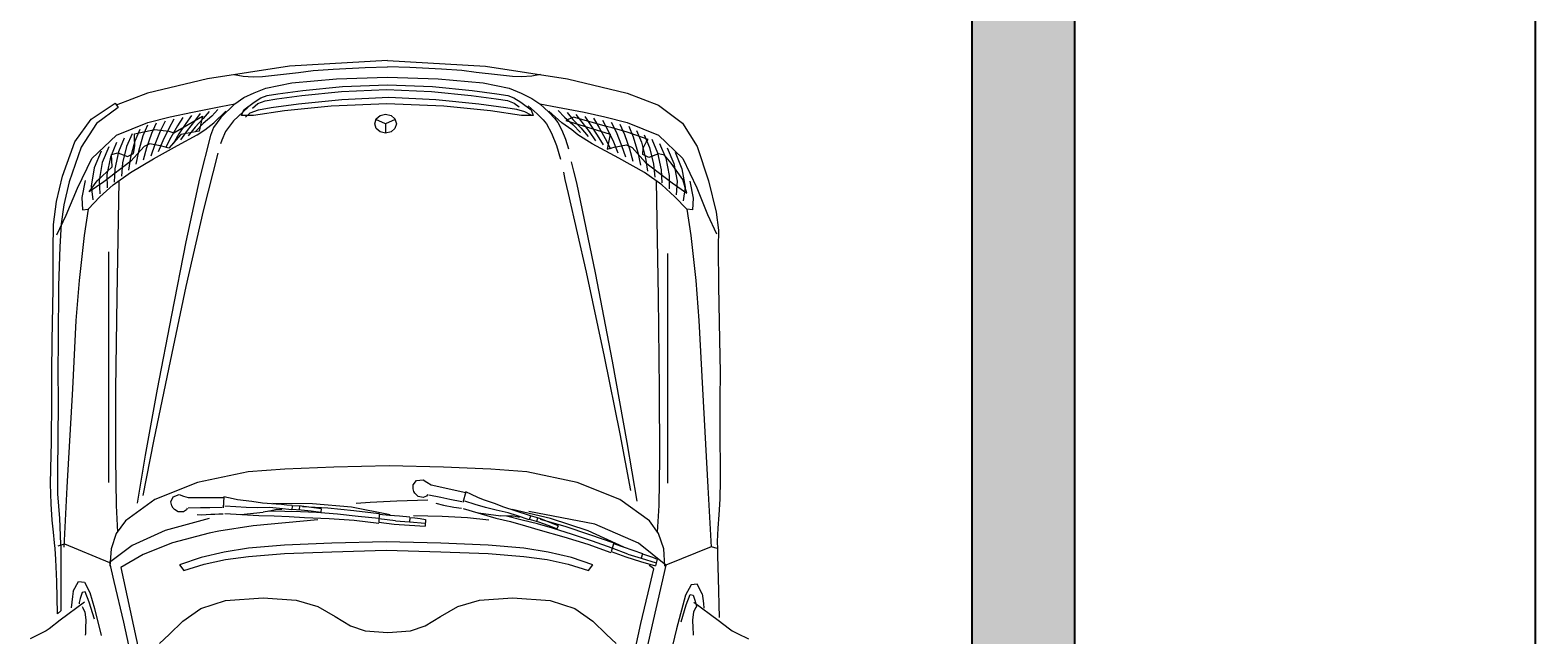
# Model space of a CAD drawing. Units: inches. Extents: x -9 to 646, y -802 to 47.
# Tile 12 of 17: x 517 to 646, y -576 to -524. Entities that reach past the tile are written whole.
import ezdxf

# ---------------------------------------------------------------- set-up
doc = ezdxf.new("R2010")
doc.units = ezdxf.units.IN
doc.header["$MEASUREMENT"] = 0
for name, color, linetype, lineweight in [('A-ANNO-DIMS', 2, 'Continuous', 18), ('A-SITE-VEHI', 8, 'Continuous', 9), ('A-WALL-PATT', 5, 'Continuous', 9), ('C-SITE', 7, 'Continuous', 25)]:
    doc.layers.add(name, color=color, linetype=linetype, lineweight=lineweight)
doc.styles.get("Standard").update_dxf_attribs({"font": 'arial.ttf'})
doc.dimstyles.get("Standard").update_dxf_attribs({"dimtxt": 0.18, "dimasz": 0.18, "dimexe": 0.18, "dimexo": 0.0625, "dimgap": 0.09, "dimtad": 0, "dimtih": 1, "dimtoh": 1, "dimdec": 0, "dimzin": 0, "dimdsep": 46, "dimlunit": 3, "dimtxsty": 'Standard', "dimcen": 0.09, "dimadec": 0, "dimazin": 0, "dimtfac": 1, "dimtdec": 0, "dimtofl": 0, "dimtmove": 0, "dimatfit": 3, "dimfxl": 1, "dimtolj": 1, "dimtzin": 0, "dimarcsym": 0})

# ---------------------------------------------------------------- blocks, each defined once
blk = doc.blocks.new('*D50')
at = {"layer": 'A-ANNO-DIMS', "color": 0, "lineweight": -2, "transparency": 16777216}
for p, q in [((606.44, 7.93), (645.8, 7.93)), ((645.62, 7.75), (645.62, -376.89)), ((645.62, -761.89), (645.62, -377.25)), ((606.44, -762.07), (645.8, -762.07))]:
    blk.add_line(p, q, dxfattribs=at)
at = {"layer": 'A-ANNO-DIMS', "color": 0, "transparency": 16777216}
for points in [[(645.59, 7.75), (645.65, 7.75), (645.62, 7.93)], [(645.59, -761.89), (645.65, -761.89), (645.62, -762.07)]]:
    blk.add_solid(points, dxfattribs=at)
at = {"layer": 'Defpoints', "color": 0, "transparency": 16777216}
for p in [(606.37, 7.93), (606.37, -762.07), (645.62, -762.07)]:
    blk.add_point(p, dxfattribs=at)
at = {"layer": 'A-ANNO-DIMS', "color": 0, "transparency": 16777216, "insert": (645.62, -377.07), "char_height": 0.18, "attachment_point": 5}
blk.add_mtext('\\A1;770', dxfattribs=at)

msp = doc.modelspace()

# ---------------------------------------------------------------- hatches: boundary and pattern name
at = {"layer": 'A-WALL-PATT'}
h = msp.add_hatch(color=256, dxfattribs=at)
h.dxf.hatch_style = 1
h.paths.add_polyline_path([(597.63, -101.57), (570.37, -101.57), (570.37, -496.07), (570.37, -511.17), (597.63, -511.17)], flags=0)
h.paths.add_polyline_path([(606.37, -101.57), (597.63, -101.57), (597.63, -511.17), (570.37, -511.17), (570.37, -513.2), (597.63, -513.2), (597.63, -712.07), (606.37, -712.07)])

# ---------------------------------------------------------------- linework, layer by layer
at = {"layer": 'A-SITE-VEHI'}
for p, q in [((539.54, -527.27), (532.56, -528.33)), ((547.88, -526.77), (539.54, -527.27)), ((541.55, -527.64), (543.27, -527.51)), ((543.27, -527.51), (545.99, -527.38)), ((545.99, -527.38), (547.88, -527.32)), ((547.88, -526.77), (556.22, -527.27)), ((549.78, -527.38), (547.88, -527.32)), ((552.5, -527.51), (549.78, -527.38)), ((554.21, -527.64), (552.5, -527.51)), ((556.22, -527.27), (563.21, -528.33)), ((532.56, -528.33), (527.46, -529.57)), ((534.84, -527.97), (535.59, -528.12)), ((535.59, -528.12), (536.46, -528.16)), ((536.46, -528.16), (537.24, -528.13)), ((537.24, -528.13), (538.52, -528.01)), ((537.52, -529.12), (539.73, -528.68)), ((538.52, -528.01), (540.31, -527.81)), ((539.73, -528.68), (543.56, -528.33)), ((540.31, -527.81), (541.55, -527.64)), ((543.56, -528.33), (547.88, -528.19)), ((544.05, -529), (547.88, -528.84)), ((547.88, -528.19), (552.21, -528.33)), ((547.88, -528.84), (551.72, -529)), ((552.21, -528.33), (556.04, -528.68)), ((555.45, -527.81), (554.21, -527.64)), ((557.25, -528.01), (555.45, -527.81)), ((556.04, -528.68), (558.25, -529.12)), ((558.52, -528.13), (557.25, -528.01)), ((559.3, -528.16), (558.52, -528.13)), ((560.18, -528.12), (559.3, -528.16)), ((560.92, -527.97), (560.18, -528.12)), ((563.21, -528.33), (568.3, -529.57)), ((527.46, -529.57), (524.8, -530.59)), ((534.9, -530.48), (535.65, -529.93)), ((535.65, -529.93), (536.53, -529.52)), ((536.53, -529.52), (537.52, -529.12)), ((536.53, -530.32), (537.11, -529.96)), ((537.11, -529.96), (537.64, -529.76)), ((537.47, -530.2), (538.47, -530.03)), ((537.64, -529.76), (538.55, -529.61)), ((538.47, -530.03), (540.6, -529.76)), ((538.55, -529.61), (540.68, -529.34)), ((540.3, -530.47), (543.99, -530.09)), ((540.6, -529.76), (543.96, -529.42)), ((540.68, -529.34), (544.05, -529)), ((543.96, -529.42), (547.8, -529.26)), ((543.99, -530.09), (548.01, -529.89)), ((547.8, -529.26), (551.64, -529.42)), ((548.01, -529.89), (552.01, -530.09)), ((551.64, -529.42), (555, -529.76)), ((551.72, -529), (555.09, -529.34)), ((552.01, -530.09), (555.66, -530.47)), ((555, -529.76), (557.13, -530.03)), ((555.09, -529.34), (557.21, -529.61)), ((557.13, -530.03), (558.1, -530.19)), ((557.21, -529.61), (558.13, -529.76)), ((558.13, -529.76), (558.65, -529.96)), ((558.25, -529.12), (559.27, -529.56)), ((558.65, -529.96), (559.23, -530.32)), ((559.27, -529.56), (560.17, -530.01)), ((560.17, -530.01), (560.87, -530.48)), ((568.3, -529.57), (570.96, -530.59)), ((522.67, -531.77), (524.69, -530.4)), ((524.95, -530.78), (523.1, -532.15)), ((524.69, -530.4), (524.95, -530.78)), ((529.39, -531.57), (531.3, -531.17)), ((531.3, -531.17), (533.71, -530.7)), ((531.95, -531.29), (531.46, -531.93)), ((532.7, -531.12), (532.19, -531.72)), ((533.45, -530.96), (532.92, -531.51)), ((533.11, -532.08), (534.13, -531.08)), ((534.9, -530.48), (533.69, -531.64)), ((533.71, -530.7), (534.9, -530.48)), ((536.04, -530.76), (534.77, -531.92)), ((535.46, -531.46), (535.66, -530.98)), ((535.66, -530.98), (536.53, -530.32)), ((535.81, -531.59), (536.19, -531.24)), ((536.19, -531.24), (536.91, -530.97)), ((536.39, -530.84), (536.85, -530.44)), ((539.12, -531.06), (536.48, -531.46)), ((536.85, -530.44), (537.47, -530.2)), ((536.91, -530.97), (537.99, -530.77)), ((537.99, -530.77), (540.3, -530.47)), ((543.09, -530.66), (539.12, -531.06)), ((547.83, -530.48), (543.09, -530.66)), ((547.26, -531.45), (547.72, -531.34)), ((547.72, -531.34), (548.19, -531.45)), ((552.69, -530.66), (547.83, -530.48)), ((556.66, -531.06), (552.69, -530.66)), ((555.66, -530.47), (557.95, -530.77)), ((559.29, -531.46), (556.66, -531.06)), ((557.95, -530.77), (558.88, -530.92)), ((558.1, -530.19), (558.68, -530.4)), ((558.68, -530.4), (559.11, -530.71)), ((558.88, -530.92), (559.54, -531.11)), ((559.23, -530.32), (560.11, -530.98)), ((559.54, -531.11), (560.09, -531.4)), ((559.86, -530.63), (560.62, -531.32)), ((560.11, -530.98), (560.3, -531.46)), ((560.62, -531.32), (561.13, -531.82)), ((560.87, -530.48), (561.62, -531.18)), ((560.87, -530.48), (562.36, -530.74)), ((561.62, -531.18), (562.12, -531.69)), ((562.73, -532.08), (561.63, -531.08)), ((562.36, -530.74), (564.62, -531.19)), ((562.43, -531.04), (562.95, -531.59)), ((563.18, -531.21), (563.68, -531.81)), ((563.93, -531.37), (564.42, -532.02)), ((564.62, -531.19), (566.38, -531.57)), ((570.96, -530.59), (573, -532.11)), ((521.28, -533.69), (522.67, -531.77)), ((523.1, -532.15), (521.81, -534.15)), ((524.82, -533.14), (527.48, -532.05)), ((526.34, -533.01), (528.08, -532.66)), ((526.79, -532.65), (526.37, -533.65)), ((527.45, -532.28), (527.07, -533.2)), ((527.48, -532.05), (529.39, -531.57)), ((528.2, -532.12), (527.8, -532.99)), ((528.08, -532.66), (529.26, -532.78)), ((528.95, -531.95), (528.53, -532.78)), ((529.26, -532.56), (528.76, -533.63)), ((529.7, -531.78), (529.26, -532.56)), ((530, -532.35), (529.44, -533.33)), ((529.7, -532.93), (532.14, -531.51)), ((530.45, -531.62), (530, -532.35)), ((530.73, -532.14), (530.13, -533.03)), ((531.2, -531.45), (530.73, -532.14)), ((531.46, -531.93), (530.82, -532.74)), ((531.51, -532.44), (530.91, -533.18)), ((532.19, -531.72), (531.51, -532.44)), ((532.2, -532.14), (531.55, -532.83)), ((531.68, -533.1), (532.34, -532.69)), ((532.14, -531.51), (531.85, -532.8)), ((532.92, -531.51), (532.2, -532.14)), ((532.34, -532.69), (533.11, -532.08)), ((533.08, -532.49), (532.81, -533.17)), ((533.69, -531.64), (533.08, -532.49)), ((534.77, -531.92), (534.1, -532.83)), ((536.48, -531.46), (535.46, -531.46)), ((546.8, -532.16), (546.93, -531.75)), ((546.93, -532.57), (546.8, -532.16)), ((547.72, -532.16), (546.9, -531.8)), ((546.93, -531.75), (547.26, -531.45)), ((547.26, -532.86), (546.93, -532.57)), ((548.55, -531.8), (547.72, -532.16)), ((547.72, -532.16), (547.72, -532.97)), ((548.19, -531.45), (548.52, -531.75)), ((548.52, -532.57), (548.19, -532.86)), ((548.52, -531.75), (548.65, -532.16)), ((548.65, -532.16), (548.52, -532.57)), ((560.3, -531.46), (559.29, -531.46)), ((561.13, -531.82), (561.42, -532.18)), ((561.42, -532.18), (561.84, -532.97)), ((562.12, -531.69), (562.4, -532.06)), ((562.4, -532.06), (562.74, -532.72)), ((563.57, -532.69), (562.73, -532.08)), ((562.95, -531.59), (563.67, -532.23)), ((563.73, -531.59), (563.07, -531.89)), ((563.07, -531.89), (566.84, -533.05)), ((564.09, -533.1), (563.57, -532.69)), ((563.67, -532.23), (564.33, -532.91)), ((563.68, -531.81), (564.36, -532.52)), ((566.52, -532.41), (563.73, -531.59)), ((564.36, -532.52), (564.96, -533.26)), ((564.42, -532.02), (565.05, -532.82)), ((564.68, -531.54), (565.15, -532.23)), ((565.15, -532.23), (565.74, -533.12)), ((565.43, -531.7), (565.88, -532.44)), ((565.88, -532.44), (566.43, -533.41)), ((566.18, -531.87), (566.61, -532.65)), ((566.38, -531.57), (568.29, -532.05)), ((567.01, -532.52), (566.52, -532.41)), ((566.61, -532.65), (567.12, -533.71)), ((566.93, -532.03), (567.35, -532.86)), ((568.29, -532.88), (567.01, -532.52)), ((567.68, -532.2), (568.08, -533.07)), ((568.29, -532.05), (570.95, -533.14)), ((568.43, -532.36), (568.81, -533.28)), ((573, -532.11), (574.26, -534.1)), ((520.22, -536.61), (521.28, -533.69)), ((522.73, -535.12), (524.82, -533.14)), ((524.82, -533.76), (524.3, -535.01)), ((525.48, -533.39), (524.99, -534.56)), ((526.14, -533.02), (525.68, -534.11)), ((526.37, -533.65), (526.01, -535.01)), ((526.36, -533.34), (526.34, -533.01)), ((526.37, -534.05), (526.36, -533.34)), ((527.07, -533.2), (526.69, -534.52)), ((527.64, -533.88), (527.16, -534.1)), ((527.8, -532.99), (527.38, -534.22)), ((528.69, -534.08), (527.64, -533.88)), ((528.07, -533.92), (527.73, -534.91)), ((528.53, -532.78), (528.07, -533.92)), ((528.76, -533.63), (528.36, -534.56)), ((529.44, -533.33), (529, -534.22)), ((529.26, -532.78), (529.7, -532.93)), ((530.29, -533.09), (529.28, -534.25)), ((530.13, -533.03), (529.64, -533.87)), ((530.01, -534.02), (531.68, -533.1)), ((530.82, -532.74), (530.27, -533.52)), ((531.85, -532.8), (530.29, -533.09)), ((532.81, -533.17), (531.88, -536.84)), ((533.79, -533.55), (533.68, -533.88)), ((534.1, -532.83), (533.79, -533.55)), ((547.72, -532.97), (547.26, -532.86)), ((548.19, -532.86), (547.72, -532.97)), ((561.84, -532.97), (562.27, -534.02)), ((562.74, -532.72), (563.04, -533.47)), ((563.04, -533.47), (563.3, -534.29)), ((565.32, -533.86), (564.09, -533.1)), ((565.05, -532.82), (565.6, -533.61)), ((567.59, -535.08), (565.32, -533.86)), ((565.74, -533.12), (566.24, -533.95)), ((566.43, -533.41), (566.88, -534.3)), ((566.84, -533.05), (566.59, -534.33)), ((567.12, -533.71), (567.51, -534.65)), ((567.18, -534.16), (568.24, -533.96)), ((567.35, -532.86), (567.81, -534.01)), ((568.08, -533.07), (568.5, -534.3)), ((568.24, -533.96), (568.72, -534.18)), ((570.07, -533.49), (568.29, -532.88)), ((568.81, -533.28), (569.19, -534.6)), ((569.08, -532.74), (569.5, -533.74)), ((569.5, -533.74), (569.86, -535.09)), ((569.65, -534.24), (569.91, -533.72)), ((569.74, -533.11), (570.19, -534.19)), ((569.91, -533.72), (570.07, -533.49)), ((570.4, -533.48), (570.88, -534.64)), ((570.95, -533.14), (573.04, -535.12)), ((571.05, -533.85), (571.58, -535.1)), ((521.81, -534.15), (520.79, -537.1)), ((521.51, -537.65), (522.73, -535.12)), ((523.51, -534.5), (522.92, -535.92)), ((524.17, -534.13), (523.61, -535.47)), ((524.3, -535.01), (524, -536.49)), ((524.4, -534.77), (524.93, -534.64)), ((524.44, -535.84), (524.4, -534.77)), ((524.99, -534.56), (524.67, -535.99)), ((524.93, -534.64), (525.74, -534.95)), ((525.68, -534.11), (525.34, -535.5)), ((525.74, -534.95), (526.25, -534.69)), ((526.01, -535.01), (525.84, -536.11)), ((526, -536.32), (527.96, -535.16)), ((527.16, -534.1), (526.03, -535.36)), ((526.25, -534.69), (526.37, -534.05)), ((526.69, -534.52), (526.45, -535.6)), ((527.38, -534.22), (527.09, -535.26)), ((527.96, -535.16), (530.01, -534.02)), ((529.28, -534.25), (528.69, -534.08)), ((533.44, -534.66), (532.19, -539.57)), ((562.27, -534.02), (562.61, -535.19)), ((566.59, -534.33), (567.18, -534.16)), ((569.76, -536.32), (567.59, -535.08)), ((567.81, -534.01), (568.15, -534.99)), ((568.5, -534.3), (568.79, -535.34)), ((568.72, -534.18), (569.85, -535.45)), ((569.19, -534.6), (569.42, -535.69)), ((569.63, -534.78), (569.65, -534.24)), ((570.14, -535.03), (569.63, -534.78)), ((569.86, -535.09), (570.03, -536.19)), ((570.95, -534.72), (570.14, -535.03)), ((570.19, -534.19), (570.53, -535.59)), ((570.88, -534.64), (571.2, -536.08)), ((571.47, -534.85), (570.95, -534.72)), ((572.03, -535.52), (571.47, -534.85)), ((571.58, -535.1), (571.88, -536.57)), ((571.71, -534.22), (572.27, -535.55)), ((572.37, -534.59), (572.96, -536.01)), ((573.04, -535.12), (574.22, -537.63)), ((574.26, -534.1), (575.22, -537.03)), ((522.92, -535.92), (522.66, -537.47)), ((523.16, -537.02), (524.44, -535.84)), ((523.61, -535.47), (523.33, -536.98)), ((526.03, -535.36), (523.74, -537.1)), ((524, -536.49), (524.02, -537.62)), ((524.52, -537.37), (526, -536.32)), ((524.67, -535.99), (524.63, -537.12)), ((525.34, -535.5), (525.24, -536.61)), ((562.86, -536.29), (563, -536.9)), ((563.54, -535.4), (563.73, -536.21)), ((563.73, -536.21), (563.97, -537.2)), ((571.24, -537.37), (569.76, -536.32)), ((569.85, -535.45), (572.13, -537.18)), ((570.53, -535.59), (570.64, -536.7)), ((571.2, -536.08), (571.25, -537.2)), ((573.02, -536.91), (572.03, -535.52)), ((572.27, -535.55), (572.55, -537.06)), ((572.96, -536.01), (573.22, -537.56)), ((519.7, -538.78), (520.22, -536.61)), ((520.79, -537.1), (520.32, -539.05)), ((520.54, -539.95), (521.51, -537.65)), ((522.16, -536.99), (521.86, -538.45)), ((522.5, -537.97), (523.16, -537.02)), ((523.74, -537.1), (522.5, -537.97)), ((522.66, -537.47), (522.8, -538.63)), ((523.33, -536.98), (523.41, -538.13)), ((523.41, -538.38), (524.52, -537.37)), ((525.02, -537.03), (524.84, -546.91)), ((531.88, -536.84), (530.73, -542.2)), ((563, -536.9), (563.14, -537.5)), ((563.14, -537.5), (563.28, -538.1)), ((563.97, -537.2), (564.16, -538.01)), ((570.75, -537.03), (570.93, -546.91)), ((572.36, -538.38), (571.24, -537.37)), ((571.88, -536.57), (571.86, -537.71)), ((572.13, -537.18), (573.38, -538.06)), ((572.55, -537.06), (572.46, -538.21)), ((573.38, -538.06), (573.02, -536.91)), ((573.22, -537.56), (573.07, -538.71)), ((573.62, -537.04), (573.91, -538.49)), ((574.22, -537.63), (575.12, -539.88)), ((575.22, -537.03), (575.88, -539.69)), ((519.44, -540.75), (519.7, -538.78)), ((520.32, -539.05), (520.11, -540.68)), ((521.86, -538.45), (521.91, -539.48)), ((522.4, -539.43), (523.41, -538.38)), ((563.28, -538.1), (564.8, -544.78)), ((564.16, -538.01), (565.58, -544.86)), ((573.37, -539.43), (572.36, -538.38)), ((573.91, -538.49), (573.85, -539.48)), ((519.73, -541.61), (520.54, -539.95)), ((521.91, -539.48), (522.4, -539.43)), ((522.4, -539.43), (522.06, -541.68)), ((532.19, -539.57), (530.73, -546)), ((573.37, -539.43), (573.71, -541.68)), ((573.85, -539.48), (573.37, -539.43)), ((575.12, -539.88), (575.9, -541.52)), ((575.88, -539.69), (576.07, -541.23)), ((519.42, -542.92), (519.44, -540.75)), ((520.11, -540.68), (519.98, -542.64)), ((522.06, -541.68), (521.63, -545.5)), ((573.71, -541.68), (574.13, -545.5)), ((576.07, -541.23), (576.04, -542.65)), ((519.42, -546.18), (519.42, -542.92)), ((519.98, -542.64), (519.89, -545.97)), ((530.73, -542.2), (529.49, -548.44)), ((576.04, -542.65), (576.06, -545.98)), ((524.16, -562.69), (524.16, -543.07)), ((571.75, -562.75), (571.75, -543.21)), ((521.63, -545.5), (521.36, -548.92)), ((564.8, -544.78), (566.33, -551.97)), ((565.58, -544.86), (567.01, -552.38)), ((574.13, -545.5), (574.4, -548.92)), ((519.35, -550.63), (519.42, -546.18)), ((519.89, -545.97), (519.85, -550.56)), ((530.73, -546), (529.27, -552.9)), ((576.06, -545.98), (576.15, -550.56)), ((524.84, -546.91), (524.74, -554.74)), ((570.93, -546.91), (571.03, -554.74)), ((521.36, -548.92), (521.06, -554.72)), ((529.49, -548.44), (528.29, -554.76)), ((574.4, -548.92), (574.71, -554.72)), ((519.31, -553.34), (519.35, -550.63)), ((519.85, -550.56), (519.83, -553.34)), ((576.15, -550.56), (576.2, -553.34)), ((529.27, -552.9), (527.98, -559.19)), ((566.33, -551.97), (567.66, -558.54)), ((567.01, -552.38), (568.26, -559.29)), ((519.3, -555.67), (519.31, -553.34)), ((519.83, -553.34), (519.84, -555.66)), ((576.2, -553.34), (576.19, -555.6)), ((519.27, -559.24), (519.3, -555.67)), ((519.84, -555.66), (519.83, -559.21)), ((521.06, -554.72), (520.6, -563.08)), ((524.74, -554.74), (524.72, -560.62)), ((528.29, -554.76), (527.27, -560.36)), ((571.03, -554.74), (571.05, -560.62)), ((574.71, -554.72), (575.17, -563.08)), ((576.19, -555.6), (576.18, -559.03)), ((519.22, -561.53), (519.27, -559.24)), ((519.83, -559.21), (519.8, -561.49)), ((527.98, -559.19), (527.07, -563.8)), ((567.66, -558.54), (568.58, -563.38)), ((568.26, -559.29), (569.11, -564.28)), ((576.18, -559.03), (576.2, -561.26)), ((524.72, -560.62), (524.78, -564.65)), ((527.27, -560.36), (526.58, -564.45)), ((571.05, -560.62), (570.99, -564.65)), ((519.2, -562.81), (519.22, -561.53)), ((519.8, -561.49), (519.8, -563.66)), ((536.02, -561.8), (531.72, -562.69)), ((539.14, -561.56), (536.02, -561.8)), ((543.32, -561.4), (539.14, -561.56)), ((548.03, -561.28), (543.32, -561.4)), ((552.67, -561.4), (548.03, -561.28)), ((556.7, -561.56), (552.67, -561.4)), ((559.75, -561.8), (556.7, -561.56)), ((564.04, -562.69), (559.75, -561.8)), ((576.2, -561.26), (576.22, -562.49)), ((519.24, -564.51), (519.2, -562.81)), ((520.6, -563.08), (520.33, -568.19)), ((531.72, -562.69), (528.09, -564.15)), ((550.08, -562.89), (550.36, -562.52)), ((550.08, -563.24), (550.08, -562.89)), ((550.14, -563.46), (550.08, -563.24)), ((550.23, -563.61), (550.14, -563.46)), ((550.36, -562.52), (550.92, -562.46)), ((550.92, -562.46), (551.23, -562.68)), ((551.23, -562.68), (551.6, -562.88)), ((551.6, -562.88), (554.55, -563.54)), ((554.56, -563.49), (554.29, -564.41)), ((555.03, -563.71), (554.56, -563.49)), ((567.67, -564.15), (564.04, -562.69)), ((575.17, -563.08), (575.44, -568.19)), ((576.22, -562.49), (576.18, -564.11)), ((519.34, -565.9), (519.24, -564.51)), ((519.8, -563.66), (519.96, -565.77)), ((524.78, -564.65), (524.91, -566.93)), ((528.09, -564.15), (525.57, -565.95)), ((529.45, -564.33), (529.64, -563.91)), ((529.52, -564.67), (529.45, -564.33)), ((529.64, -564.88), (529.52, -564.67)), ((529.64, -563.91), (530.16, -563.72)), ((530.16, -563.72), (530.51, -563.87)), ((530.51, -563.87), (530.93, -563.97)), ((530.93, -563.97), (533.94, -563.96)), ((533.95, -563.91), (533.89, -564.86)), ((534.34, -563.99), (533.95, -563.91)), ((534.97, -564.77), (534.03, -564.7)), ((534.74, -564.08), (534.34, -563.99)), ((535.13, -564.16), (534.74, -564.08)), ((535.87, -564.83), (534.97, -564.77)), ((536.35, -564.32), (535.13, -564.16)), ((537.26, -564.44), (536.35, -564.32)), ((538.4, -564.54), (537.26, -564.44)), ((541.49, -564.5), (538.13, -564.47)), ((538.85, -564.57), (538.4, -564.54)), ((539.31, -564.62), (538.85, -564.57)), ((539.76, -564.65), (539.31, -564.62)), ((539.77, -564.68), (539.74, -565.02)), ((540.58, -564.72), (539.75, -564.67)), ((540.39, -564.71), (540.36, -565)), ((541.42, -564.82), (540.58, -564.72)), ((540.64, -564.75), (542.82, -564.85)), ((544.83, -564.8), (541.49, -564.5)), ((546.42, -564.41), (545.22, -564.47)), ((548.69, -564.29), (546.42, -564.41)), ((551.32, -564.21), (548.69, -564.29)), ((550.49, -563.88), (550.23, -563.61)), ((550.92, -563.97), (550.49, -563.88)), ((551.22, -563.87), (550.92, -563.97)), ((551.27, -563.78), (551.22, -563.87)), ((551.32, -563.74), (551.27, -563.78)), ((552.43, -563.97), (551.41, -563.76)), ((552.01, -564.46), (552.66, -564.61)), ((553.19, -564.13), (552.43, -563.97)), ((552.66, -564.61), (553.55, -564.78)), ((554.21, -564.35), (553.19, -564.13)), ((553.55, -564.78), (554.18, -564.89)), ((555.36, -564.56), (554.46, -564.28)), ((555.59, -563.98), (555.03, -563.71)), ((556.23, -564.82), (555.36, -564.56)), ((556.06, -564.18), (555.59, -563.98)), ((556.99, -564.49), (556.06, -564.18)), ((557.8, -564.8), (556.99, -564.49)), ((570.2, -565.95), (567.67, -564.15)), ((570.99, -564.65), (570.86, -566.93)), ((576.18, -564.11), (576.09, -565.46)), ((519.45, -566.93), (519.34, -565.9)), ((519.96, -565.77), (520.05, -567.93)), ((525.57, -565.95), (524.8, -567.03)), ((532.7, -565.76), (528.97, -566.79)), ((529.76, -565), (529.64, -564.88)), ((530.07, -565.2), (529.76, -565)), ((530.51, -565.19), (530.07, -565.2)), ((530.78, -565.03), (530.51, -565.19)), ((530.8, -564.93), (530.78, -565.03)), ((530.84, -564.88), (530.8, -564.93)), ((531.97, -564.86), (530.93, -564.88)), ((531.68, -565.43), (532.07, -565.44)), ((532.75, -564.84), (531.97, -564.86)), ((532.07, -565.44), (532.46, -565.42)), ((532.46, -565.42), (532.85, -565.39)), ((533.8, -564.83), (532.75, -564.84)), ((532.85, -565.39), (533.2, -565.38)), ((533.2, -565.38), (533.54, -565.37)), ((533.54, -565.37), (533.89, -565.36)), ((534.03, -565.34), (536.93, -565.51)), ((535.41, -565.42), (537.3, -565.23)), ((536.82, -564.84), (535.87, -564.83)), ((541.96, -565.87), (536.45, -566.37)), ((537.85, -564.83), (536.82, -564.84)), ((536.93, -565.51), (538.23, -565.52)), ((537.83, -565.14), (537.3, -565.23)), ((539.14, -565.17), (537.79, -565.14)), ((538.36, -565.03), (537.83, -565.14)), ((538.69, -564.9), (537.85, -564.83)), ((538.23, -565.52), (539.53, -565.59)), ((538.9, -564.99), (538.36, -565.03)), ((539.74, -565.02), (538.69, -564.9)), ((540.49, -565.19), (539.14, -565.17)), ((539.53, -565.59), (540.83, -565.66)), ((539.72, -564.96), (540.55, -565.01)), ((541.84, -565.24), (540.49, -565.19)), ((540.55, -565.01), (541.39, -565.11)), ((540.83, -565.66), (542.93, -565.77)), ((541.39, -565.11), (542.21, -565.22)), ((542.24, -564.94), (541.42, -564.82)), ((543.62, -565.39), (541.84, -565.24)), ((542.24, -564.94), (542.2, -565.22)), ((542.82, -564.85), (545.01, -565.08)), ((542.93, -565.77), (545.06, -565.91)), ((545.39, -565.58), (543.62, -565.39)), ((548.12, -565.46), (544.83, -564.8)), ((545.01, -565.08), (547.19, -565.32)), ((545.06, -565.91), (547.14, -566.15)), ((547.16, -565.76), (545.39, -565.58)), ((547.19, -565.32), (547.14, -566.08)), ((548.58, -565.96), (547.15, -565.78)), ((547.18, -565.38), (548.05, -565.47)), ((548.05, -565.47), (548.92, -565.54)), ((548.58, -565.96), (549.75, -566.05)), ((548.92, -565.54), (549.78, -565.63)), ((549.79, -565.66), (549.75, -566.05)), ((549.75, -566.05), (551.1, -566.15)), ((549.79, -565.66), (550.23, -565.71)), ((552.54, -565.59), (550.09, -565.54)), ((550.23, -565.71), (550.68, -565.76)), ((550.68, -565.76), (551.12, -565.83)), ((551.12, -565.83), (551.09, -566.4)), ((554.7, -565.71), (552.54, -565.59)), ((554.32, -564.91), (557.11, -565.72)), ((556.53, -565.89), (554.7, -565.71)), ((555.65, -565.29), (557.53, -565.54)), ((557.15, -565.04), (556.23, -564.82)), ((557.11, -565.72), (558.37, -566.02)), ((558.16, -565.27), (557.15, -565.04)), ((558.07, -565.56), (557.53, -565.54)), ((558.76, -565.11), (557.8, -564.8)), ((559.34, -565.89), (558.03, -565.55)), ((558.61, -565.57), (558.07, -565.56)), ((558.96, -565.53), (558.16, -565.27)), ((558.37, -566.02), (559.63, -566.38)), ((561.78, -565.76), (558.51, -564.98)), ((559.14, -565.66), (558.61, -565.57)), ((559.19, -565.24), (558.76, -565.11)), ((559.95, -565.87), (558.96, -565.53)), ((559.63, -565.38), (559.19, -565.24)), ((560.65, -566.21), (559.34, -565.89)), ((560.06, -565.52), (559.63, -565.38)), ((565.53, -566.25), (559.92, -565.16)), ((560.06, -565.55), (559.95, -565.87)), ((559.95, -565.81), (560.75, -566.05)), ((560.85, -565.77), (560.05, -565.54)), ((560.66, -565.72), (560.57, -566)), ((560.75, -566.05), (561.54, -566.33)), ((561.64, -566.06), (560.85, -565.77)), ((560.89, -565.81), (563, -566.4)), ((562.41, -566.37), (561.64, -566.06)), ((564.97, -566.8), (561.78, -565.76)), ((570.96, -567.03), (570.2, -565.95)), ((576.09, -565.46), (576, -566.59)), ((519.54, -567.82), (519.45, -566.93)), ((524.8, -567.03), (524.36, -568.35)), ((528.97, -566.79), (526.15, -568.05)), ((532.7, -567.02), (529.59, -567.84)), ((533.54, -566.83), (532.7, -567.02)), ((536.45, -566.37), (533.54, -566.83)), ((547.14, -566.08), (548.46, -566.23)), ((548.46, -566.23), (549.77, -566.33)), ((549.77, -566.33), (551.09, -566.4)), ((559.63, -566.38), (560.88, -566.75)), ((561.95, -566.57), (560.65, -566.21)), ((560.88, -566.75), (562.89, -567.33)), ((561.54, -566.33), (562.32, -566.63)), ((563.65, -567.11), (561.95, -566.57)), ((562.41, -566.37), (562.31, -566.63)), ((562.89, -567.33), (564.94, -567.94)), ((563, -566.4), (565.08, -567.12)), ((565.33, -567.7), (563.65, -567.11)), ((568.02, -568.19), (564.97, -566.8)), ((565.08, -567.12), (567.15, -567.84)), ((569.25, -567.86), (565.53, -566.25)), ((571.41, -568.35), (570.96, -567.03)), ((576, -566.59), (575.96, -567.72)), ((519.59, -568.3), (519.54, -567.82)), ((519.64, -569.24), (519.59, -568.3)), ((519.84, -568.09), (520.38, -567.92)), ((520.05, -567.93), (520.07, -567.97)), ((520.07, -567.97), (520.09, -568.02)), ((520.08, -568.56), (520.07, -570.28)), ((520.09, -568.08), (520.08, -568.56)), ((520.09, -568.02), (520.09, -568.08)), ((520.38, -567.92), (524.23, -569.5)), ((526.15, -568.05), (524.23, -569.5)), ((524.36, -568.35), (524.26, -569.82)), ((529.59, -567.84), (527.08, -568.82)), ((533.99, -568.61), (532.02, -569.09)), ((536.06, -568.27), (533.99, -568.61)), ((539.11, -568.03), (536.06, -568.27)), ((543.14, -567.87), (539.11, -568.03)), ((539.11, -568.74), (543.14, -568.59)), ((547.78, -567.75), (543.14, -567.87)), ((543.14, -568.59), (547.78, -568.46)), ((552.42, -567.87), (547.78, -567.75)), ((547.78, -568.46), (552.42, -568.59)), ((556.45, -568.03), (552.42, -567.87)), ((552.42, -568.59), (556.45, -568.74)), ((559.5, -568.27), (556.45, -568.03)), ((561.57, -568.61), (559.5, -568.27)), ((563.55, -569.09), (561.57, -568.61)), ((564.94, -567.94), (566.91, -568.64)), ((567.02, -568.27), (565.33, -567.7)), ((567.15, -567.84), (566.93, -568.58)), ((566.93, -568.58), (568.18, -569.01)), ((568.36, -568.78), (567.01, -568.29)), ((567.13, -567.9), (567.95, -568.18)), ((567.95, -568.18), (568.78, -568.45)), ((568.78, -568.45), (569.6, -568.73)), ((571.59, -569.73), (569.25, -567.86)), ((571.51, -569.82), (571.41, -568.35)), ((575.44, -568.16), (571.59, -569.73)), ((575.98, -568.32), (575.44, -568.16)), ((575.96, -567.72), (575.98, -568.35)), ((575.98, -568.35), (575.99, -568.94)), ((519.73, -571.12), (519.64, -569.24)), ((524.23, -569.5), (524.6, -571.11)), ((527.08, -568.82), (525.18, -569.94)), ((532.02, -569.09), (530.18, -569.7)), ((530.18, -569.7), (530.55, -570.19)), ((530.55, -570.19), (532.29, -569.64)), ((532.29, -569.64), (534.09, -569.26)), ((534.09, -569.26), (536.06, -568.99)), ((536.06, -568.99), (539.11, -568.74)), ((556.45, -568.74), (559.5, -568.99)), ((559.5, -568.99), (561.47, -569.26)), ((561.47, -569.26), (563.27, -569.64)), ((563.27, -569.64), (565.01, -570.19)), ((565.38, -569.7), (563.55, -569.09)), ((565.01, -570.19), (565.38, -569.7)), ((568.18, -569.01), (569.44, -569.41)), ((568.36, -568.78), (569.48, -569.13)), ((569.44, -569.41), (570.71, -569.78)), ((569.6, -568.76), (569.48, -569.13)), ((569.48, -569.13), (570.77, -569.53)), ((569.6, -568.76), (570.03, -568.91)), ((570.03, -568.91), (570.45, -569.06)), ((570.3, -569.85), (570.17, -569.76)), ((570.43, -569.94), (570.3, -569.85)), ((570.45, -569.06), (570.86, -569.22)), ((570.86, -569.22), (570.71, -569.78)), ((571.59, -569.73), (571.22, -571.34)), ((575.99, -568.94), (576.04, -570.83)), ((519.8, -573.88), (519.73, -571.12)), ((520.07, -570.28), (520.09, -573.63)), ((521.14, -571.94), (521.58, -571.11)), ((521.58, -571.11), (522.08, -571.17)), ((522.08, -571.17), (522.55, -572.05)), ((524.6, -571.11), (525.4, -574.57)), ((525.18, -569.94), (528.59, -585.53)), ((570.21, -571.5), (570.56, -570.04)), ((570.56, -570.04), (570.43, -569.94)), ((576.04, -570.83), (576.14, -574.19)), ((521.07, -572.4), (521.02, -572.87)), ((521.14, -571.94), (521.07, -572.4)), ((521.9, -572.05), (521.73, -572.56)), ((522.15, -572.01), (521.9, -572.05)), ((522.49, -572.88), (522.15, -572.01)), ((522.55, -572.05), (522.94, -573.43)), ((569.47, -574.7), (570.21, -571.5)), ((571.22, -571.34), (570.42, -574.81)), ((573.27, -572.28), (572.5, -575.15)), ((573.74, -571.41), (573.27, -572.28)), ((573.33, -573.11), (573.67, -572.24)), ((573.67, -572.24), (573.92, -572.28)), ((574.24, -571.34), (573.74, -571.41)), ((573.92, -572.28), (574.09, -572.8)), ((574.68, -572.17), (574.24, -571.34)), ((574.68, -572.17), (574.74, -572.57)), ((520.09, -573.63), (519.8, -573.88)), ((522.1, -572.87), (520.02, -574.42)), ((521.02, -572.87), (520.97, -573.35)), ((521.65, -572.9), (521.63, -573.02)), ((521.73, -572.56), (521.65, -572.9)), ((521.88, -573.25), (521.96, -573.37)), ((521.96, -573.37), (522.12, -573.74)), ((522.12, -573.74), (522.21, -574.39)), ((522.93, -574.32), (522.49, -572.88)), ((522.94, -573.43), (523.51, -575.71)), ((530.45, -574.49), (532, -573.41)), ((532, -573.41), (534.09, -572.75)), ((534.09, -572.75), (537.3, -572.52)), ((537.3, -572.52), (540.11, -572.71)), ((540.11, -572.71), (541.95, -573.25)), ((541.95, -573.25), (543.44, -574.11)), ((552.39, -574.11), (553.89, -573.25)), ((553.89, -573.25), (555.72, -572.71)), ((555.72, -572.71), (558.53, -572.52)), ((558.53, -572.52), (561.74, -572.75)), ((561.74, -572.75), (563.83, -573.41)), ((563.83, -573.41), (565.38, -574.49)), ((572.89, -574.56), (573.33, -573.11)), ((573.95, -573.74), (573.87, -574.39)), ((574.11, -573.37), (573.95, -573.74)), ((573.98, -572.87), (576.05, -574.42)), ((574.09, -572.8), (574.17, -573.13)), ((574.19, -573.25), (574.11, -573.37)), ((574.17, -573.13), (574.19, -573.25)), ((574.74, -572.57), (574.79, -572.98)), ((574.79, -572.98), (574.83, -573.39)), ((520.02, -574.42), (519.07, -575.14)), ((522.21, -574.39), (522.19, -575.09)), ((525.4, -574.57), (526.13, -577.85)), ((529.3, -575.62), (530.45, -574.49)), ((543.44, -574.11), (544.73, -574.9)), ((544.73, -574.9), (545.99, -575.33)), ((549.84, -575.33), (551.1, -574.9)), ((551.1, -574.9), (552.39, -574.11)), ((565.38, -574.49), (566.53, -575.62)), ((568.77, -577.83), (569.47, -574.7)), ((570.42, -574.81), (569.69, -578.08)), ((573.87, -574.39), (573.88, -575.09)), ((576.05, -574.42), (577, -575.14)), ((518.38, -575.54), (517.46, -575.99)), ((518.84, -575.32), (518.38, -575.54)), ((519.07, -575.14), (518.84, -575.32)), ((522.17, -575.54), (522.15, -575.69)), ((522.19, -575.09), (522.17, -575.54)), ((528.47, -576.39), (529.3, -575.62)), ((545.99, -575.33), (547.92, -575.45)), ((547.92, -575.45), (549.84, -575.33)), ((566.53, -575.62), (567.36, -576.39)), ((572.5, -575.15), (571.45, -579.49)), ((573.88, -575.09), (573.91, -575.54)), ((573.91, -575.54), (573.92, -575.69)), ((577, -575.14), (577.23, -575.32)), ((577.23, -575.32), (577.69, -575.54)), ((577.69, -575.54), (578.61, -575.99))]:
    msp.add_line(p, q, dxfattribs=at)
at = {"layer": 'C-SITE'}
for p, q in [((606.37, -101.57), (606.37, -762.07)), ((597.63, -513.2), (597.63, -762.07))]:
    msp.add_line(p, q, dxfattribs=at)

# ---------------------------------------------------------------- dimensions: what is measured, and where the dimension line sits
at = {"layer": 'A-ANNO-DIMS'}
dim = msp.add_linear_dim(base=(645.62, -762.07), p1=(606.37, 7.93), p2=(606.37, -762.07), angle=90, dimstyle='Standard', override={"dimdec": 0, "dimlfac": 1, "dimrnd": 0, "dimzin": 0, "dimdsep": 46, "dimlunit": 2}, dxfattribs=at)
dim.commit()
dim.dimension.update_dxf_attribs({"geometry": '*D50', "text_midpoint": (645.62, -377.07)})

doc.saveas('drawing.dxf')
